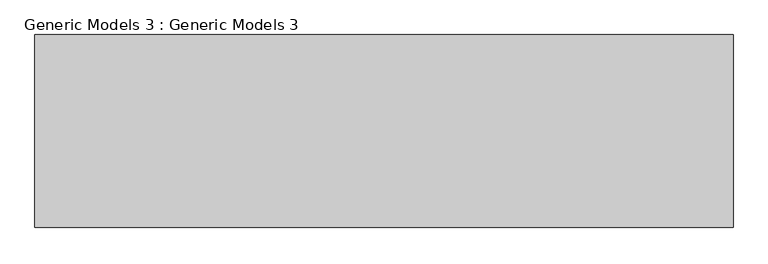
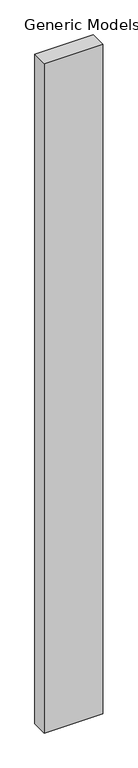
"""IFC4 building model written with IfcOpenShell, lengths in millimetres: proxy geometry, Generic Models 3 : Generic Models 3."""

from ifc_helpers import new_model, si_unit, frame, origin, place, context, project, spatial, polyline, outline, extrude, source, transform, mapped, element, save


def generic_models_3_generic_models_3_f60183ce(model_context):
    return source(origin(), model_context, "Body", "SweptSolid", [
        extrude(outline(polyline([(13598.5361222, -32.3497958), (13598.5361222, 328.1471911), (14902.2061109, 328.1471911), (14902.2061109, -32.3497958), (13598.5361222, -32.3497958)])), frame((0.0, 0.0, 2810.1257279), z_axis=(0.0, 0.0, 1.0), x_axis=(1.0, 0.0, 0.0)), (0.0, 0.0, 1.0), 15806.9265941),
    ])


if __name__ == "__main__":
    model = new_model("IFC4")
    model_context = context("Model", 3, world=origin())
    ifc_project = project(units=[si_unit("LENGTHUNIT", "METRE", prefix="MILLI")], contexts=[model_context])
    site = spatial("IfcSite", under=ifc_project)
    building = spatial("IfcBuilding", under=site)
    placement = place(None, origin())
    generic_models_3_generic_models_3_shape = generic_models_3_generic_models_3_f60183ce(model_context)
    element("IfcBuildingElementProxy", 1, Name="Generic Models 3 : Generic Models 3", ObjectType="Generic Models 3 : Generic Models 3", at=placement, inside=building, context=model_context, shape_type="MappedRepresentation", body=[
        mapped(generic_models_3_generic_models_3_shape, transform((0.0, 0.0, 0.0), x_axis=(1.0, 0.0, 0.0), y_axis=(0.0, 1.0, 0.0), z_axis=(0.0, 0.0, 1.0))),
    ])
    save(model, "model.ifc")
